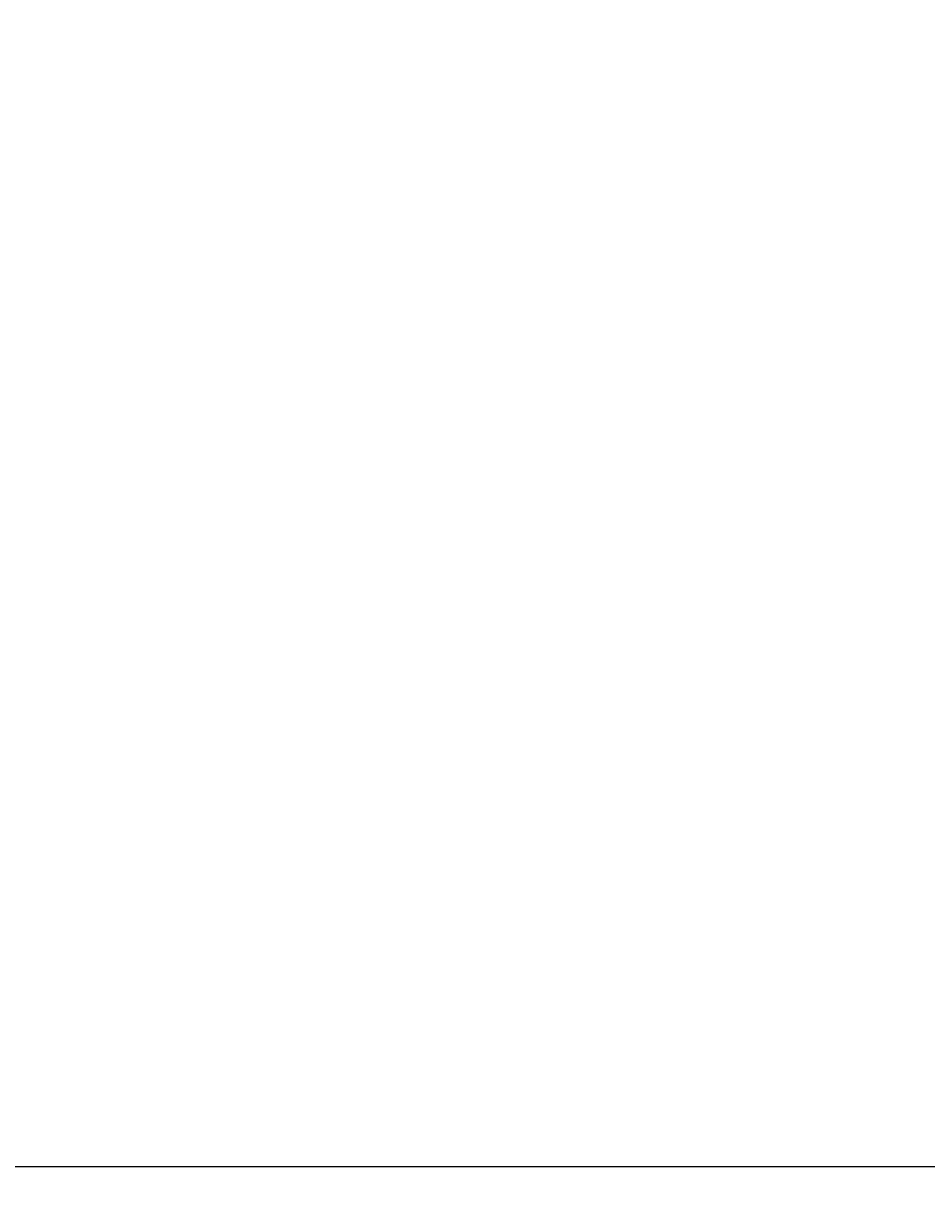
# Model space of a CAD drawing. Units: inches. Extents: x 35362 to 73946, y 43607 to 67532.
# Tile 111 of 134: x 50905 to 50977, y 48969 to 49061. Entities that reach past the tile are written whole.
import ezdxf

# ---------------------------------------------------------------- set-up
doc = ezdxf.new("R2010")
doc.units = ezdxf.units.IN
doc.header["$MEASUREMENT"] = 0
doc.layers.add('A-ANNO-DIMS', color=2, linetype='Continuous', lineweight=18)
doc.styles.get("Standard").update_dxf_attribs({"font": 'arial.ttf'})
doc.dimstyles.get("Standard").update_dxf_attribs({"dimtxt": 0.18, "dimasz": 0.18, "dimexe": 0.18, "dimexo": 0.0625, "dimgap": 0.09, "dimtad": 0, "dimtih": 1, "dimtoh": 1, "dimdec": 4, "dimzin": 0, "dimdsep": 46, "dimtxsty": 'Standard', "dimcen": 0.09, "dimadec": 0, "dimazin": 0, "dimtfac": 1, "dimtdec": 4, "dimtofl": 0, "dimtmove": 0, "dimatfit": 3, "dimfxl": 1, "dimtolj": 1, "dimtzin": 0, "dimarcsym": 0})

# ---------------------------------------------------------------- blocks, each defined once
blk = doc.blocks.new('*D11')
at = {"layer": 'A-ANNO-DIMS', "color": 0, "lineweight": -2, "transparency": 16777216}
for p, q in [((47978.665, 56028.774), (47978.665, 43606.679)), ((53109.76, 56028.774), (53109.76, 43606.679)), ((47978.845, 43606.859), (50543.871, 43606.859)), ((53109.58, 43606.859), (50544.554, 43606.859))]:
    blk.add_line(p, q, dxfattribs=at)
at = {"layer": 'A-ANNO-DIMS', "color": 0, "transparency": 16777216}
for points in [[(47978.845, 43606.889), (47978.845, 43606.829), (47978.665, 43606.859)], [(53109.58, 43606.889), (53109.58, 43606.829), (53109.76, 43606.859)]]:
    blk.add_solid(points, dxfattribs=at)
at = {"layer": 'Defpoints', "color": 0, "transparency": 16777216}
for p in [(47978.665, 56028.836), (53109.76, 56028.836), (53109.76, 43606.859)]:
    blk.add_point(p, dxfattribs=at)
at = {"layer": 'A-ANNO-DIMS', "color": 0, "transparency": 16777216, "insert": (50544.212, 43606.859), "char_height": 0.18, "attachment_point": 5}
blk.add_mtext('\\A1;5131', dxfattribs=at)
blk = doc.blocks.new('*D13')
at = {"layer": 'A-ANNO-DIMS', "color": 0, "lineweight": -2, "transparency": 16777216}
for p, q in [((48373.492, 51694.025), (48373.492, 43606.679)), ((51029.043, 51694.025), (51029.043, 43606.679)), ((48373.672, 43606.859), (49700.802, 43606.859)), ((51028.863, 43606.859), (49701.733, 43606.859))]:
    blk.add_line(p, q, dxfattribs=at)
at = {"layer": 'A-ANNO-DIMS', "color": 0, "transparency": 16777216}
for points in [[(48373.672, 43606.889), (48373.672, 43606.829), (48373.492, 43606.859)], [(51028.863, 43606.889), (51028.863, 43606.829), (51029.043, 43606.859)]]:
    blk.add_solid(points, dxfattribs=at)
at = {"layer": 'Defpoints', "color": 0, "transparency": 16777216}
for p in [(48373.492, 51694.087), (51029.043, 51694.087), (51029.043, 43606.859)]:
    blk.add_point(p, dxfattribs=at)
at = {"layer": 'A-ANNO-DIMS', "color": 0, "transparency": 16777216, "insert": (49701.267, 43606.859), "char_height": 0.18, "attachment_point": 5}
blk.add_mtext('\\A1;2655.6', dxfattribs=at)
blk = doc.blocks.new('*D17')
at = {"layer": 'A-ANNO-DIMS', "color": 0, "lineweight": -2, "transparency": 16777216}
for p, q in [((49923.307, 61293.224), (49923.307, 43606.679)), ((51913.931, 61293.224), (51913.931, 43606.679)), ((49923.487, 43606.859), (50918.164, 43606.859)), ((51913.751, 43606.859), (50919.074, 43606.859))]:
    blk.add_line(p, q, dxfattribs=at)
at = {"layer": 'A-ANNO-DIMS', "color": 0, "transparency": 16777216}
for points in [[(49923.487, 43606.889), (49923.487, 43606.829), (49923.307, 43606.859)], [(51913.751, 43606.889), (51913.751, 43606.829), (51913.931, 43606.859)]]:
    blk.add_solid(points, dxfattribs=at)
at = {"layer": 'Defpoints', "color": 0, "transparency": 16777216}
for p in [(49923.307, 61293.286), (51913.931, 61293.286), (51913.931, 43606.859)]:
    blk.add_point(p, dxfattribs=at)
at = {"layer": 'A-ANNO-DIMS', "color": 0, "transparency": 16777216, "insert": (50918.619, 43606.859), "char_height": 0.18, "attachment_point": 5}
blk.add_mtext('\\A1;1990.6', dxfattribs=at)
blk = doc.blocks.new('*D67')
at = {"layer": 'A-ANNO-DIMS', "color": 0, "lineweight": -2, "transparency": 16777216}
for p, q in [((56873.539, 53351.529), (35361.769, 53351.529)), ((35361.949, 53351.349), (35361.949, 49400.893)), ((35361.949, 45450.074), (35361.949, 49400.53)), ((53793.575, 45449.894), (35361.769, 45449.894))]:
    blk.add_line(p, q, dxfattribs=at)
at = {"layer": 'A-ANNO-DIMS', "color": 0, "transparency": 16777216}
for points in [[(35361.919, 53351.349), (35361.979, 53351.349), (35361.949, 53351.529)], [(35361.919, 45450.074), (35361.979, 45450.074), (35361.949, 45449.894)]]:
    blk.add_solid(points, dxfattribs=at)
at = {"layer": 'Defpoints', "color": 0, "transparency": 16777216}
for p in [(35361.949, 53351.529), (56873.602, 53351.529), (53793.638, 45449.894)]:
    blk.add_point(p, dxfattribs=at)
at = {"layer": 'A-ANNO-DIMS', "color": 0, "transparency": 16777216, "insert": (35361.949, 49400.712), "char_height": 0.18, "attachment_point": 5}
blk.add_mtext('\\A1;7901.6', dxfattribs=at)
blk = doc.blocks.new('*D84')
at = {"layer": 'A-ANNO-DIMS', "color": 0, "lineweight": -2, "transparency": 16777216}
for p, q in [((55540.235, 49259.935), (35361.769, 49259.935)), ((35361.949, 49259.755), (35361.949, 49115.139)), ((35361.949, 48970.16), (35361.949, 49114.776)), ((55540.235, 48969.98), (35361.769, 48969.98))]:
    blk.add_line(p, q, dxfattribs=at)
at = {"layer": 'A-ANNO-DIMS', "color": 0, "transparency": 16777216}
for points in [[(35361.919, 49259.755), (35361.979, 49259.755), (35361.949, 49259.935)], [(35361.919, 48970.16), (35361.979, 48970.16), (35361.949, 48969.98)]]:
    blk.add_solid(points, dxfattribs=at)
at = {"layer": 'Defpoints', "color": 0, "transparency": 16777216}
for p in [(35361.949, 49259.935), (55540.297, 49259.935), (55540.297, 48969.98)]:
    blk.add_point(p, dxfattribs=at)
at = {"layer": 'A-ANNO-DIMS', "color": 0, "transparency": 16777216, "insert": (35361.949, 49114.957), "char_height": 0.18, "attachment_point": 5}
blk.add_mtext('\\A1;289.96', dxfattribs=at)
blk = doc.blocks.new('*D86')
at = {"layer": 'A-ANNO-DIMS', "color": 0, "lineweight": -2, "transparency": 16777216}
for p, q in [((51285.532, 49320.079), (35361.769, 49320.079)), ((35361.949, 49319.899), (35361.949, 49120.261)), ((35361.949, 48920.259), (35361.949, 49119.897)), ((51285.532, 48920.079), (35361.769, 48920.079))]:
    blk.add_line(p, q, dxfattribs=at)
at = {"layer": 'A-ANNO-DIMS', "color": 0, "transparency": 16777216}
for points in [[(35361.919, 49319.899), (35361.979, 49319.899), (35361.949, 49320.079)], [(35361.919, 48920.259), (35361.979, 48920.259), (35361.949, 48920.079)]]:
    blk.add_solid(points, dxfattribs=at)
at = {"layer": 'Defpoints', "color": 0, "transparency": 16777216}
for p in [(35361.949, 49320.079), (51285.595, 49320.079), (51285.595, 48920.079)]:
    blk.add_point(p, dxfattribs=at)
at = {"layer": 'A-ANNO-DIMS', "color": 0, "transparency": 16777216, "insert": (35361.949, 49120.079), "char_height": 0.18, "attachment_point": 5}
blk.add_mtext('\\A1;400.0', dxfattribs=at)
blk = doc.blocks.new('*D107')
at = {"layer": 'A-ANNO-DIMS', "color": 0, "lineweight": -2, "transparency": 16777216}
for p, q in [((50139.563, 59850.014), (50139.563, 43606.679)), ((51320.813, 59850.014), (51320.813, 43606.679)), ((50139.743, 43606.859), (50729.733, 43606.859)), ((51320.633, 43606.859), (50730.643, 43606.859))]:
    blk.add_line(p, q, dxfattribs=at)
at = {"layer": 'A-ANNO-DIMS', "color": 0, "transparency": 16777216}
for points in [[(50139.743, 43606.889), (50139.743, 43606.829), (50139.563, 43606.859)], [(51320.633, 43606.889), (51320.633, 43606.829), (51320.813, 43606.859)]]:
    blk.add_solid(points, dxfattribs=at)
at = {"layer": 'Defpoints', "color": 0, "transparency": 16777216}
for p in [(50139.563, 59850.077), (51320.813, 59850.077), (51320.813, 43606.859)]:
    blk.add_point(p, dxfattribs=at)
at = {"layer": 'A-ANNO-DIMS', "color": 0, "transparency": 16777216, "insert": (50730.188, 43606.859), "char_height": 0.18, "attachment_point": 5}
blk.add_mtext('\\A1;1181.3', dxfattribs=at)

msp = doc.modelspace()

# ---------------------------------------------------------------- dimensions: what is measured, and where the dimension line sits
at = {"layer": 'A-ANNO-DIMS'}
for base, p1, p2, override, picture, middle in [((51913.931, 43606.859), (49923.307, 61293.286), (51913.931, 61293.286), {"dimdec": 1, "dimlfac": 1, "dimrnd": 0, "dimzin": 0, "dimdsep": 46, "dimlunit": 2}, '*D17', (50918.619, 43606.859)), ((51320.8133, 43606.859), (50139.5627, 59850.0769), (51320.8133, 59850.0769), {"dimdec": 1, "dimlfac": 1, "dimrnd": 0, "dimzin": 0, "dimdsep": 46, "dimlunit": 2}, '*D107', (50730.188, 43606.859)), ((53109.76, 43606.859), (47978.665, 56028.836), (53109.76, 56028.836), {"dimdec": 0, "dimlfac": 1, "dimrnd": 0, "dimzin": 0, "dimdsep": 46, "dimlunit": 2}, '*D11', (50544.212, 43606.859)), ((51029.043, 43606.859), (48373.492, 51694.087), (51029.043, 51694.087), {"dimdec": 1, "dimlfac": 1, "dimrnd": 0, "dimzin": 0, "dimdsep": 46, "dimlunit": 2}, '*D13', (49701.267, 43606.859))]:
    dim = msp.add_linear_dim(base=base, p1=p1, p2=p2, dimstyle='Standard', override=override, dxfattribs=at)
    dim.commit()
    dim.dimension.update_dxf_attribs({"geometry": picture, "text_midpoint": middle})
for base, p1, p2, override, picture, middle in [((35361.949, 53351.529), (53793.638, 45449.894), (56873.602, 53351.529), {"dimdec": 1, "dimlfac": 1, "dimrnd": 0, "dimzin": 0, "dimdsep": 46, "dimlunit": 2}, '*D67', (35361.949, 49400.712)), ((35361.949, 49320.079), (51285.595, 48920.079), (51285.595, 49320.079), {"dimdec": 1, "dimlfac": 1, "dimrnd": 0, "dimzin": 0, "dimdsep": 46, "dimlunit": 2}, '*D86', (35361.949, 49120.079)), ((35361.9491, 49259.9353), (55540.2972, 48969.9796), (55540.2972, 49259.9353), {"dimdec": 2, "dimlfac": 1, "dimrnd": 0, "dimzin": 0, "dimdsep": 46, "dimlunit": 2}, '*D84', (35361.9491, 49114.9575))]:
    dim = msp.add_linear_dim(base=base, p1=p1, p2=p2, angle=90, dimstyle='Standard', override=override, dxfattribs=at)
    dim.commit()
    dim.dimension.update_dxf_attribs({"geometry": picture, "text_midpoint": middle})

doc.saveas('drawing.dxf')
